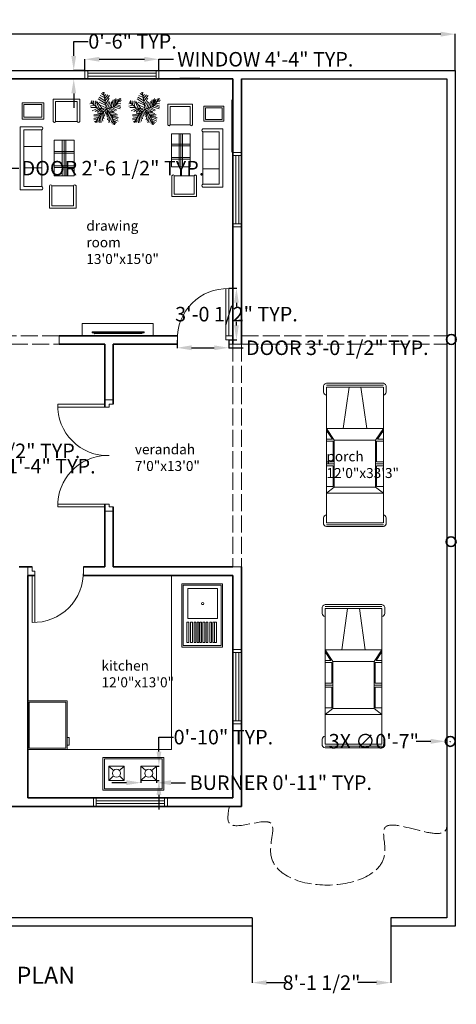
# Model space of a CAD drawing. Units: inches. Extents: x 29 to 4581, y 6 to 2196.
# Tile 3 of 3: x 4274 to 4581, y 1506 to 2196. Entities that reach past the tile are written whole.
import ezdxf

# ---------------------------------------------------------------- set-up
doc = ezdxf.new("R2010")
doc.units = ezdxf.units.IN
doc.header["$MEASUREMENT"] = 0
doc.linetypes.add('ACAD_ISO02W100', pattern=[15, 12, -3])
for name, color, linetype, lineweight in [('A-ANNO-DIMS', 2, 'Continuous', 18), ('A-ANNO-TEXT', 7, 'Continuous', 25), ('A-DOOR', 3, 'Continuous', 18), ('A-EQPM', 9, 'Continuous', 18), ('A-FLOR-CASE', 8, 'Continuous', 18), ('A-FLOR-FIXT', 9, 'Continuous', 18), ('A-GLAZ', 4, 'Continuous', 18), ('A-ROOF-OVHD', 8, 'ACAD_ISO02W100', 18), ('A-WALL', 7, 'Continuous', 35), ('A-WALL-OVHD', 8, 'ACAD_ISO02W100', 18), ('C-PKNG-VEHI', 8, 'Continuous', 13), ('C-PROP', 8, 'Continuous', 25), ('L-PLNT', 3, 'Continuous', 13)]:
    doc.layers.add(name, color=color, linetype=linetype, lineweight=lineweight)
for name, color, linetype, lineweight, true_color in [('A-AREA-IDEN', 41, 'Continuous', 18, 0xf4ee51), ('A-COLS', 240, 'Continuous', 35, 0xed1f24), ('A-FURN', 31, 'Continuous', 18, 0xfecc66)]:
    doc.layers.add(name, color=color, linetype=linetype, lineweight=lineweight, true_color=true_color)
doc.styles.get("Standard").update_dxf_attribs({"font": 'arial.ttf'})
doc.dimstyles.get("Standard").update_dxf_attribs({"dimtxt": 10.18, "dimasz": 10.18, "dimexe": 0.18, "dimexo": 0.0625, "dimgap": 0.09, "dimtad": 0, "dimtih": 1, "dimtoh": 1, "dimdec": 0, "dimzin": 0, "dimdsep": 46, "dimlunit": 3, "dimtxsty": 'Standard', "dimcen": 0.09, "dimadec": 0, "dimazin": 0, "dimtfac": 1, "dimtdec": 0, "dimtofl": 0, "dimtmove": 0, "dimatfit": 3, "dimfxl": 1, "dimtolj": 1, "dimtzin": 0, "dimarcsym": 0})

# ---------------------------------------------------------------- blocks, each defined once
blk = doc.blocks.new('*U4')
for p, q in [((-3.665, 19.273), (-27.574, 35.527)), ((-5.114, 28.097), (-24.676, 40.636)), ((-7.288, 39.707), (-21.778, 46.673)), ((-8.737, 47.138), (-17.069, 52.711)), ((-10.186, 53.64), (-13.084, 55.962)), ((0, 0), (-10.5, 57)), ((-9.099, 51.782), (-6.563, 55.962)), ((-7.65, 43.423), (-2.578, 49.46)), ((-5.839, 35.992), (4.667, 48.067)), ((-5.114, 27.632), (10.463, 46.673)), ((-2.941, 16.486), (8.652, 37.85)), ((27, 9), (48, 36)), ((27.127, 9.056), (31.112, 35.992)), ((38.719, 34.134), (41.979, 28.561)), ((44.153, 36.456), (45.239, 32.741)), ((-47.498, 19.737), (-55.83, 18.344)), ((-40.615, 13.7), (-55.105, 10.913)), ((-31.5, 4.5), (-52.5, 25.5)), ((-33.37, 6.269), (-52.207, 5.34)), ((-48.585, 21.131), (-49.309, 29.026)), ((-28.299, 3.483), (-47.86, -5.805)), ((-43.513, 28.561), (-42.427, 15.558)), ((-38.442, 26.239), (-34.819, 7.663)), ((-21.416, 3.018), (-38.079, -8.128)), ((-35.544, 28.097), (-24.314, 3.947)), ((0, 0), (-31.5, 4.5)), ((-14.533, 2.09), (-30.834, 25.31)), ((-15.982, 2.09), (-30.11, -9.521)), ((-24.314, 23.917), (-2.941, 13.7)), ((0, 0), (-22.5, -19.5)), ((-6.563, 1.161), (-21.416, -8.128)), ((-20.691, 13.7), (-1.129, 4.876)), ((-1.129, 6.734), (9.014, 26.704)), ((0, 0), (27, 9)), ((0, 0), (18, -22.5)), ((3.942, 1.625), (11.187, 24.381)), ((6.478, 1.625), (26.04, -8.592)), ((10.101, 3.483), (17.708, 26.239)), ((11.187, 3.483), (30.749, -5.805)), ((16.259, 5.805), (23.142, 31.348)), ((18.07, 5.805), (35.096, -3.483)), ((22.055, 7.198), (27.489, 32.277)), ((24.229, 7.663), (46.688, 1.625)), ((29.662, 12.307), (48.137, 6.269)), ((31.836, 30.883), (32.561, 16.486)), ((33.285, 16.486), (48.862, 10.913)), ((35.096, 32.741), (37.27, 22.524)), ((36.183, 19.737), (48.137, 17.88)), ((40.53, 25.775), (48.862, 24.846)), ((43.791, 29.954), (51.036, 30.883)), ((-17.431, -15.094), (-42.789, -18.809)), ((-28.299, -29.026), (-42.789, -31.348)), ((-24.314, -21.596), (-42.427, -22.06)), ((-26.849, -26.24), (-40.253, -25.775)), ((-22.5, -19.5), (-37.5, -45)), ((-15.257, -12.772), (-30.11, -12.772)), ((-29.023, -30.884), (-27.936, -43.887)), ((-25.038, -23.918), (-22.865, -45.281)), ((-20.691, -18.345), (-17.793, -44.352)), ((-6.563, -5.805), (-19.967, -9.985)), ((-17.069, -15.094), (-12.721, -40.172)), ((-13.446, -11.378), (-8.737, -32.741)), ((-9.461, -8.592), (-6.201, -23.453)), ((-4.752, -3.483), (-3.665, -14.629)), ((2.493, -3.019), (-1.491, -20.202)), ((1.769, -2.555), (24.229, -9.521)), ((5.029, -6.27), (2.131, -25.775)), ((9.014, -11.378), (3.58, -35.992)), ((14.085, -16.951), (6.478, -40.172)), ((7.565, -9.056), (32.198, -14.629)), ((18.07, -22.524), (8.289, -45.745)), ((12.274, -15.094), (36.907, -18.809)), ((20.244, -30.419), (15.897, -44.816)), ((16.259, -19.738), (36.183, -22.989)), ((18, -22.5), (27, -52.5)), ((18.433, -22.524), (40.53, -29.026)), ((19.157, -25.311), (38.719, -33.206)), ((21.331, -32.741), (39.081, -40.636)), ((-30.834, -34.135), (-42.427, -35.528)), ((-34.457, -39.708), (-40.978, -42.494)), ((-32.646, -36.921), (-31.921, -44.352)), ((22.78, -37.85), (19.519, -48.532)), ((22.78, -38.314), (34.372, -44.816)), ((24.591, -45.745), (23.142, -50.854)), ((24.591, -43.423), (30.749, -47.603)), ((26.764, -49.925), (28.213, -50.854))]:
    blk.add_line(p, q)
blk = doc.blocks.new('*U6')
for p, q in [((5.4, 42.3), (12.1, 42.3)), ((189.7, 42.3), (183, 42.3)), ((0.1, -0.4), (0.1, 38.3)), ((2.8, -0.4), (2.8, 38.3)), ((5.4, 38.3), (16.1, 38.3)), ((5.4, -0.4), (5.4, 38.2)), ((16.1, 38.3), (180.3, 38.3)), ((61.5, -0.4), (61.5, 38.3)), ((61.5, 38.3), (77.5, 27.6)), ((64.2, 38.3), (76.2, 30.3)), ((76.2, 30.3), (76.2, 38.3)), ((77.5, 27.6), (141.6, 27.6)), ((77.5, -0.4), (77.5, 27.6)), ((78.9, 38.3), (78.9, 29)), ((78.9, 29), (106.9, 29)), ((106.9, 29), (106.9, 38.3)), ((109.6, 27.6), (109.6, 38.3)), ((112.3, 38.3), (112.3, 29)), ((112.3, 29), (140.3, 29)), ((140.3, 29), (140.3, 38.3)), ((141.6, 27.6), (149.6, 38.3)), ((141.6, -0.4), (141.6, 27.6)), ((149.6, -0.4), (149.6, 38.3)), ((189.7, 38.3), (179, 38.3)), ((189.7, -0.4), (189.7, 38.2)), ((192.4, -0.4), (192.4, 38.3)), ((195, -0.4), (195, 38.3)), ((5.4, 7.6), (61.5, 15.6)), ((0.1, -0.4), (0.1, -39.2)), ((2.8, -0.4), (2.8, -39.1)), ((5.4, -0.4), (5.4, -39.1)), ((5.4, -8.4), (61.5, -16.4)), ((61.5, -0.4), (61.5, -39.1)), ((77.5, -0.4), (77.5, -28.5)), ((141.6, -0.4), (141.6, -28.5)), ((149.6, -0.4), (149.6, -39.1)), ((189.7, -0.4), (189.7, -39.1)), ((192.4, -0.4), (192.4, -39.1)), ((195, -0.4), (195, -39.2)), ((5.4, -39.1), (16.1, -39.1)), ((16.1, -39.1), (180.3, -39.1)), ((61.5, -39.1), (77.5, -28.5)), ((64.2, -39.1), (76.2, -31.1)), ((76.2, -31.1), (76.2, -39.1)), ((77.5, -28.5), (141.6, -28.5)), ((78.9, -39.1), (78.9, -29.8)), ((78.9, -29.8), (106.9, -29.8)), ((106.9, -29.8), (106.9, -39.1)), ((109.6, -28.5), (109.6, -39.1)), ((112.3, -29.8), (140.3, -29.8)), ((112.3, -39.1), (112.3, -29.8)), ((140.3, -29.8), (140.3, -39.1)), ((141.6, -28.5), (149.6, -39.1)), ((189.7, -39.1), (179, -39.1)), ((5.4, -43.1), (12.1, -43.1)), ((189.7, -43.1), (183, -43.1))]:
    blk.add_line(p, q)
for centre, radius, start, end in [((5.1, 37.3), 5.06, 85.6455, 168.0943), ((11.5, 37.6), 4.72, 8.1301, 81.87), ((183.7, 37.6), 4.72, 98.13, 171.8699), ((190.1, 37.3), 5.06, 11.9057, 94.3545), ((5.1, -38.1), 5.06, 191.9057, 274.3545), ((11.5, -38.5), 4.72, 278.13, 351.8699), ((183.7, -38.5), 4.72, 188.1301, 261.87), ((190.1, -38.1), 5.06, 265.6455, 348.0943)]:
    blk.add_arc(centre, radius, start, end)
blk = doc.blocks.new('*D7')
at = {"layer": 'A-ANNO-DIMS', "color": 0, "lineweight": -2, "transparency": 16777216}
for p, q in [((3871.98, 2160.26), (3871.98, 2185.77)), ((3882.16, 2185.59), (4217.25, 2185.59)), ((4569.8, 2185.59), (4234.7, 2185.59)), ((4579.98, 2160.26), (4579.98, 2185.77))]:
    blk.add_line(p, q, dxfattribs=at)
at = {"layer": 'A-ANNO-DIMS', "color": 0, "transparency": 16777216}
for points in [[(3882.16, 2187.28), (3882.16, 2183.89), (3871.98, 2185.59)], [(4569.8, 2187.28), (4569.8, 2183.89), (4579.98, 2185.59)]]:
    blk.add_solid(points, dxfattribs=at)
at = {"layer": 'Defpoints', "color": 0, "transparency": 16777216}
for p in [(4579.98, 2185.59), (3871.98, 2160.2), (4579.98, 2160.2)]:
    blk.add_point(p, dxfattribs=at)
at = {"layer": 'A-ANNO-DIMS', "color": 0, "transparency": 16777216, "insert": (4225.98, 2185.59), "char_height": 10.18, "attachment_point": 5}
blk.add_mtext("\\A1;59'", dxfattribs=at)
blk = doc.blocks.new('DOOR-36IN')
for p, q in [((34.01, 0), (34.01, 36)), ((36.01, 3), (36.01, 36)), ((34.01, 0), (36.01, 0))]:
    blk.add_line(p, q)
blk.add_arc((35.01, 1), 35.01, 88.36342, 181.63658)
blk = doc.blocks.new('DOOR-36IN-PAIRED-LEAF')
for p, q in [((36.01, 2), (0.01, 2)), ((36.01, 2), (36.01, 0)), ((33.01, 0), (0.01, 0))]:
    blk.add_line(p, q)
blk.add_arc((35.01, 1), 35.01, 91.63658, 181.63658)
blk = doc.blocks.new('WIN-48')
for p, q in [((0, 6), (0, 0)), ((2, 6), (2, 0)), ((2, 4), (50, 4)), ((2, 2), (50, 2)), ((50, 6), (50, 0)), ((52, 6), (52, 0))]:
    blk.add_line(p, q)
blk = doc.blocks.new('HOB-BURNER')
for p, q in [((0, 9.96), (3.37, 6.89)), ((10.94, 9.96), (7.57, 6.89)), ((0, 0), (3.37, 3.07)), ((10.94, 0), (7.57, 3.07))]:
    blk.add_line(p, q)
blk.add_lwpolyline([(0, 9.96), (10.94, 9.96), (10.94, 0), (0, 0)], close=True)
blk.add_circle((5.47, 4.98), 2.84)
blk = doc.blocks.new('PORCH-POST-ROUND')
blk.add_circle((3.47, 3.47), 3.47)
blk = doc.blocks.new('*D22')
at = {"layer": 'A-ANNO-DIMS', "color": 0, "lineweight": -2, "transparency": 16777216}
for p, q in [((4226.82, 1911.89), (4226.82, 1922.07)), ((4229.23, 1901.71), (4226.64, 1901.71)), ((4229.23, 1885.22), (4226.64, 1885.22)), ((4226.82, 1875.04), (4226.82, 1864.86))]:
    blk.add_line(p, q, dxfattribs=at)
at = {"layer": 'A-ANNO-DIMS', "color": 0, "transparency": 16777216}
for points in [[(4225.13, 1911.89), (4228.52, 1911.89), (4226.82, 1901.71)], [(4225.13, 1875.04), (4228.52, 1875.04), (4226.82, 1885.22)]]:
    blk.add_solid(points, dxfattribs=at)
at = {"layer": 'Defpoints', "color": 0, "transparency": 16777216}
for p in [(4229.3, 1901.71), (4226.82, 1885.22), (4229.3, 1885.22)]:
    blk.add_point(p, dxfattribs=at)
at = {"layer": 'A-ANNO-DIMS', "color": 0, "transparency": 16777216, "insert": (4226.82, 1893.47), "char_height": 10.18, "attachment_point": 5}
blk.add_mtext('\\A1;DINING CHAIR 1\'-4 1/2" TYP.', dxfattribs=at)
blk = doc.blocks.new('*D23')
at = {"layer": 'A-ANNO-DIMS', "color": 0, "lineweight": -2, "transparency": 16777216}
for p, q in [((4229.3, 1885.16), (4229.3, 1882.56)), ((4245.51, 1885.16), (4245.51, 1882.56)), ((4219.12, 1882.74), (4208.94, 1882.74)), ((4255.69, 1882.74), (4265.87, 1882.74))]:
    blk.add_line(p, q, dxfattribs=at)
at = {"layer": 'A-ANNO-DIMS', "color": 0, "transparency": 16777216}
for points in [[(4219.12, 1884.44), (4219.12, 1881.05), (4229.3, 1882.74)], [(4255.69, 1884.44), (4255.69, 1881.05), (4245.51, 1882.74)]]:
    blk.add_solid(points, dxfattribs=at)
at = {"layer": 'Defpoints', "color": 0, "transparency": 16777216}
for p in [(4229.3, 1885.22), (4245.51, 1885.22), (4245.51, 1882.74)]:
    blk.add_point(p, dxfattribs=at)
at = {"layer": 'A-ANNO-DIMS', "color": 0, "transparency": 16777216, "insert": (4296.5, 1882.74), "char_height": 10.18, "attachment_point": 5}
blk.add_mtext('\\A1;1\'-4" TYP.', dxfattribs=at)
blk = doc.blocks.new('*D24')
at = {"layer": 'A-ANNO-DIMS', "color": 0, "lineweight": -2, "transparency": 16777216}
for p, q in [((4384.7, 1971.13), (4384.7, 1965.58)), ((4420.98, 1971.13), (4420.98, 1965.58)), ((4394.88, 1965.76), (4410.8, 1965.76)), ((4420.98, 1965.76), (4431.16, 1965.76))]:
    blk.add_line(p, q, dxfattribs=at)
at = {"layer": 'A-ANNO-DIMS', "color": 0, "transparency": 16777216}
for points in [[(4394.88, 1967.45), (4394.88, 1964.06), (4384.7, 1965.76)], [(4410.8, 1967.45), (4410.8, 1964.06), (4420.98, 1965.76)]]:
    blk.add_solid(points, dxfattribs=at)
at = {"layer": 'Defpoints', "color": 0, "transparency": 16777216}
for p in [(4384.7, 1971.2), (4420.98, 1971.2), (4420.98, 1965.76)]:
    blk.add_point(p, dxfattribs=at)
at = {"layer": 'A-ANNO-DIMS', "color": 0, "transparency": 16777216, "insert": (4497.19, 1965.76), "char_height": 10.18, "attachment_point": 5}
blk.add_mtext('\\A1;DOOR 3\'-0 1/2" TYP.', dxfattribs=at)
blk = doc.blocks.new('*D25')
at = {"layer": 'A-ANNO-DIMS', "color": 0, "lineweight": -2, "transparency": 16777216}
for p, q in [((4421.04, 2007.47), (4426.6, 2007.47)), ((4426.42, 1997.29), (4426.42, 1994.69)), ((4426.42, 1981.38), (4426.42, 1983.98)), ((4421.04, 1971.2), (4426.6, 1971.2))]:
    blk.add_line(p, q, dxfattribs=at)
at = {"layer": 'A-ANNO-DIMS', "color": 0, "transparency": 16777216}
for points in [[(4424.72, 1997.29), (4428.11, 1997.29), (4426.42, 2007.47)], [(4424.72, 1981.38), (4428.11, 1981.38), (4426.42, 1971.2)]]:
    blk.add_solid(points, dxfattribs=at)
at = {"layer": 'Defpoints', "color": 0, "transparency": 16777216}
for p in [(4420.98, 2007.47), (4426.42, 2007.47), (4420.98, 1971.2)]:
    blk.add_point(p, dxfattribs=at)
at = {"layer": 'A-ANNO-DIMS', "color": 0, "transparency": 16777216, "insert": (4426.42, 1989.33), "char_height": 10.18, "attachment_point": 5}
blk.add_mtext('\\A1;3\'-0 1/2" TYP.', dxfattribs=at)
blk = doc.blocks.new('*D26')
at = {"layer": 'A-ANNO-DIMS', "color": 0, "lineweight": -2, "transparency": 16777216}
for p, q in [((4319.98, 2160.26), (4319.98, 2168.18)), ((4330.16, 2168), (4361.8, 2168)), ((4371.98, 2160.26), (4371.98, 2168.18)), ((4371.98, 2168), (4382.16, 2168))]:
    blk.add_line(p, q, dxfattribs=at)
at = {"layer": 'A-ANNO-DIMS', "color": 0, "transparency": 16777216}
for points in [[(4330.16, 2169.69), (4330.16, 2166.3), (4319.98, 2168)], [(4361.8, 2169.69), (4361.8, 2166.3), (4371.98, 2168)]]:
    blk.add_solid(points, dxfattribs=at)
at = {"layer": 'Defpoints', "color": 0, "transparency": 16777216}
for p in [(4371.98, 2168), (4319.98, 2160.2), (4371.98, 2160.2)]:
    blk.add_point(p, dxfattribs=at)
at = {"layer": 'A-ANNO-DIMS', "color": 0, "transparency": 16777216, "insert": (4446.66, 2168), "char_height": 10.18, "attachment_point": 5}
blk.add_mtext('\\A1;WINDOW 4\'-4" TYP.', dxfattribs=at)
blk = doc.blocks.new('*D27')
at = {"layer": 'A-ANNO-DIMS', "color": 0, "lineweight": -2, "transparency": 16777216}
for p, q in [((4312.18, 2170.38), (4312.18, 2180.56)), ((4312.18, 2180.56), (4322.36, 2180.56)), ((4319.91, 2160.2), (4312, 2160.2)), ((4319.91, 2154.2), (4312, 2154.2)), ((4312.18, 2144.02), (4312.18, 2133.84))]:
    blk.add_line(p, q, dxfattribs=at)
at = {"layer": 'A-ANNO-DIMS', "color": 0, "transparency": 16777216}
for points in [[(4310.48, 2170.38), (4313.87, 2170.38), (4312.18, 2160.2)], [(4310.48, 2144.02), (4313.87, 2144.02), (4312.18, 2154.2)]]:
    blk.add_solid(points, dxfattribs=at)
at = {"layer": 'Defpoints', "color": 0, "transparency": 16777216}
for p in [(4312.18, 2160.2), (4319.98, 2160.2), (4319.98, 2154.2)]:
    blk.add_point(p, dxfattribs=at)
at = {"layer": 'A-ANNO-DIMS', "color": 0, "transparency": 16777216, "insert": (4353.47, 2180.56), "char_height": 10.18, "attachment_point": 5}
blk.add_mtext('\\A1;0\'-6" TYP.', dxfattribs=at)
blk = doc.blocks.new('*D28')
at = {"layer": 'A-ANNO-DIMS', "color": 0, "lineweight": -2, "transparency": 16777216}
for p, q in [((4263.52, 2081.47), (4263.52, 2091.65)), ((4263.52, 2091.65), (4273.7, 2091.65)), ((4259.04, 2081.47), (4263.7, 2081.47)), ((4263.52, 2061.38), (4263.52, 2071.29)), ((4259.04, 2051.2), (4263.7, 2051.2))]:
    blk.add_line(p, q, dxfattribs=at)
at = {"layer": 'A-ANNO-DIMS', "color": 0, "transparency": 16777216}
for points in [[(4261.82, 2071.29), (4265.21, 2071.29), (4263.52, 2081.47)], [(4261.82, 2061.38), (4265.21, 2061.38), (4263.52, 2051.2)]]:
    blk.add_solid(points, dxfattribs=at)
at = {"layer": 'Defpoints', "color": 0, "transparency": 16777216}
for p in [(4258.98, 2081.47), (4263.52, 2081.47), (4258.98, 2051.2)]:
    blk.add_point(p, dxfattribs=at)
at = {"layer": 'A-ANNO-DIMS', "color": 0, "transparency": 16777216, "insert": (4339.73, 2091.65), "char_height": 10.18, "attachment_point": 5}
blk.add_mtext('\\A1;DOOR 2\'-6 1/2" TYP.', dxfattribs=at)
blk = doc.blocks.new('*D44')
at = {"layer": 'A-ANNO-DIMS', "color": 0, "lineweight": -2, "transparency": 16777216}
for p, q in [((4349.23, 1660.87), (4339.05, 1660.87)), ((4359.41, 1662.45), (4359.41, 1660.69)), ((4370.35, 1662.45), (4370.35, 1660.69)), ((4380.53, 1660.87), (4390.71, 1660.87))]:
    blk.add_line(p, q, dxfattribs=at)
at = {"layer": 'A-ANNO-DIMS', "color": 0, "transparency": 16777216}
for points in [[(4349.23, 1662.57), (4349.23, 1659.18), (4359.41, 1660.87)], [(4380.53, 1662.57), (4380.53, 1659.18), (4370.35, 1660.87)]]:
    blk.add_solid(points, dxfattribs=at)
at = {"layer": 'Defpoints', "color": 0, "transparency": 16777216}
for p in [(4359.41, 1662.51), (4370.35, 1662.51), (4370.35, 1660.87)]:
    blk.add_point(p, dxfattribs=at)
at = {"layer": 'A-ANNO-DIMS', "color": 0, "transparency": 16777216, "insert": (4457.56, 1660.87), "char_height": 10.18, "attachment_point": 5}
blk.add_mtext('\\A1;BURNER 0\'-11" TYP.', dxfattribs=at)
blk = doc.blocks.new('*D45')
at = {"layer": 'A-ANNO-DIMS', "color": 0, "lineweight": -2, "transparency": 16777216}
for p, q in [((4371.99, 1682.65), (4371.99, 1692.83)), ((4371.99, 1692.83), (4382.17, 1692.83)), ((4370.41, 1672.47), (4372.17, 1672.47)), ((4370.41, 1662.51), (4372.17, 1662.51)), ((4371.99, 1652.33), (4371.99, 1642.15))]:
    blk.add_line(p, q, dxfattribs=at)
at = {"layer": 'A-ANNO-DIMS', "color": 0, "transparency": 16777216}
for points in [[(4370.29, 1682.65), (4373.69, 1682.65), (4371.99, 1672.47)], [(4370.29, 1652.33), (4373.69, 1652.33), (4371.99, 1662.51)]]:
    blk.add_solid(points, dxfattribs=at)
at = {"layer": 'Defpoints', "color": 0, "transparency": 16777216}
for p in [(4370.35, 1672.47), (4371.99, 1672.47), (4370.35, 1662.51)]:
    blk.add_point(p, dxfattribs=at)
at = {"layer": 'A-ANNO-DIMS', "color": 0, "transparency": 16777216, "insert": (4417.24, 1692.83), "char_height": 10.18, "attachment_point": 5}
blk.add_mtext('\\A1;0\'-10" TYP.', dxfattribs=at)
blk = doc.blocks.new('*D46')
at = {"layer": 'A-ANNO-DIMS', "color": 0, "lineweight": -2, "transparency": 16777216}
for p, q in [((4437.42, 1560.13), (4437.42, 1520.52)), ((4534.84, 1560.13), (4534.84, 1520.52)), ((4447.6, 1520.7), (4460.64, 1520.7)), ((4524.66, 1520.7), (4511.62, 1520.7))]:
    blk.add_line(p, q, dxfattribs=at)
at = {"layer": 'A-ANNO-DIMS', "color": 0, "transparency": 16777216}
for points in [[(4447.6, 1522.39), (4447.6, 1519), (4437.42, 1520.7)], [(4524.66, 1522.39), (4524.66, 1519), (4534.84, 1520.7)]]:
    blk.add_solid(points, dxfattribs=at)
at = {"layer": 'Defpoints', "color": 0, "transparency": 16777216}
for p in [(4437.42, 1560.2), (4534.84, 1560.2), (4534.84, 1520.7)]:
    blk.add_point(p, dxfattribs=at)
at = {"layer": 'A-ANNO-DIMS', "color": 0, "transparency": 16777216, "insert": (4486.13, 1520.7), "char_height": 10.18, "attachment_point": 5}
blk.add_mtext('\\A1;8\'-1 1/2"', dxfattribs=at)
blk = doc.blocks.new('*D50')
at = {"layer": 'A-ANNO-DIMS', "color": 0, "lineweight": -2, "transparency": 16777216}
for p, q in [((4552.67, 1689.94), (4562.85, 1689.89)), ((4576.41, 1689.82), (4576.59, 1689.82)), ((4576.5, 1689.73), (4576.5, 1689.91))]:
    blk.add_line(p, q, dxfattribs=at)
at = {"layer": 'A-ANNO-DIMS', "color": 0, "transparency": 16777216}
blk.add_solid([(4562.86, 1691.59), (4562.85, 1688.19), (4573.03, 1689.84)], dxfattribs=at)
at = {"layer": 'Defpoints', "color": 0, "transparency": 16777216}
for p in [(4573.03, 1689.84), (4579.97, 1689.81)]:
    blk.add_point(p, dxfattribs=at)
at = {"layer": 'A-ANNO-DIMS', "color": 0, "transparency": 16777216, "insert": (4522.85, 1689.94), "char_height": 10.18, "attachment_point": 5}
blk.add_mtext('\\A1;3X ∅0\'-7"', dxfattribs=at)

msp = doc.modelspace()

# ---------------------------------------------------------------- linework, layer by layer
at = {"layer": 'A-DOOR'}
for p, q in [((4384.98, 1974.2), (4384.98, 1968.2)), ((4418.98, 1974.2), (4423.98, 1974.2)), ((4420.98, 1971.2), (4420.98, 1968.2)), ((4420.98, 1968.2), (4423.98, 1968.2)), ((4339.98, 1929.2), (4333.98, 1929.2)), ((4339.98, 1926.2), (4336.98, 1926.2)), ((4333.98, 1890.24), (4333.98, 1890.15)), ((4336.98, 1890.2), (4333.98, 1890.2)), ((4339.98, 1851.2), (4333.98, 1851.2)), ((4339.98, 1854.2), (4336.98, 1854.2)), ((4279.98, 1806.2), (4279.98, 1812.2)), ((4282.98, 1809.2), (4282.98, 1812.2)), ((4318.98, 1806.2), (4318.98, 1812.2))]:
    msp.add_line(p, q, dxfattribs=at)
at = {"layer": 'A-EQPM'}
for p, q in [((4327.52, 1976.14), (4326.64, 1975.61)), ((4326.64, 1975.61), (4360.24, 1975.67)), ((4360.24, 1975.67), (4359.23, 1976.14))]:
    msp.add_line(p, q, dxfattribs=at)
for points in [[(4318.17, 1974.2), (4368.06, 1974.2), (4368.06, 1982.86), (4318.17, 1982.86)], [(4325.24, 1976.99), (4361.61, 1976.99), (4361.61, 1976.14), (4325.24, 1976.14)], [(4279.98, 1718.34), (4307.57, 1718.34), (4307.57, 1684.14), (4279.98, 1684.14)], [(4280.98, 1717.34), (4306.57, 1717.34), (4306.57, 1685.14), (4280.98, 1685.14)], [(4307.57, 1687.9), (4307.57, 1687.9), (4307.57, 1694.82), (4307.57, 1694.82)], [(4307.57, 1687.15), (4309.1, 1687.15), (4309.1, 1692.45), (4307.57, 1692.45)], [(4332.73, 1678.63), (4375.37, 1678.63), (4375.37, 1655.6), (4332.73, 1655.6)], [(4333.73, 1677.63), (4374.37, 1677.63), (4374.37, 1656.6), (4333.73, 1656.6)]]:
    msp.add_lwpolyline(points, close=True, dxfattribs=at)
at = {"layer": 'A-FLOR-CASE'}
for p, q in [((4380.83, 1806.2), (4380.83, 1684.14)), ((4380.83, 1684.14), (4279.98, 1684.14))]:
    msp.add_line(p, q, dxfattribs=at)
at = {"layer": 'A-FLOR-FIXT'}
for points in [[(4416.67, 1800.35), (4388.04, 1800.35), (4388.04, 1755.97), (4416.67, 1755.97)], [(4415.67, 1799.35), (4389.04, 1799.35), (4389.04, 1756.97), (4415.67, 1756.97)], [(4392.31, 1796.95), (4413, 1796.95), (4413, 1775.95), (4392.31, 1775.95)], [(4392.9, 1773.39), (4391.67, 1773.39), (4391.67, 1759.08), (4392.9, 1759.08)], [(4395.46, 1773.39), (4394.23, 1773.39), (4394.23, 1759.08), (4395.46, 1759.08)], [(4397.88, 1773.39), (4396.65, 1773.39), (4396.65, 1759.08), (4397.88, 1759.08)], [(4400, 1773.39), (4398.76, 1773.39), (4398.76, 1759.08), (4400, 1759.08)], [(4401.93, 1773.39), (4400.7, 1773.39), (4400.7, 1759.08), (4401.93, 1759.08)], [(4404.13, 1773.39), (4402.9, 1773.39), (4402.9, 1759.08), (4404.13, 1759.08)], [(4406.38, 1773.39), (4405.15, 1773.39), (4405.15, 1759.08), (4406.38, 1759.08)], [(4408.97, 1773.39), (4407.74, 1773.39), (4407.74, 1759.08), (4408.97, 1759.08)], [(4411.09, 1773.39), (4409.85, 1773.39), (4409.85, 1759.08), (4411.09, 1759.08)], [(4412.32, 1773.39), (4411.09, 1773.39), (4411.09, 1759.08), (4412.32, 1759.08)]]:
    msp.add_lwpolyline(points, close=True, dxfattribs=at)
msp.add_circle((4402.65, 1786.45), 0.779, dxfattribs=at)
at = {"layer": 'A-FURN'}
for p, q in [((4386.19, 2115.79), (4386.19, 2092.65)), ((4387.37, 2115.79), (4387.37, 2092.65)), ((4388.55, 2115.79), (4388.55, 2092.65)), ((4277.28, 2106.91), (4289.76, 2106.91)), ((4304.14, 2111.39), (4304.14, 2086.31)), ((4305.42, 2111.39), (4305.42, 2086.31)), ((4306.69, 2111.39), (4306.69, 2086.31)), ((4380.91, 2108.42), (4393.84, 2108.42)), ((4380.91, 2107.24), (4393.84, 2107.24)), ((4298.4, 2103.4), (4312.43, 2103.4)), ((4298.4, 2102.12), (4312.43, 2102.12)), ((4380.91, 2099.19), (4393.84, 2099.19)), ((4414.38, 2105.01), (4402.87, 2105.01)), ((4277.28, 2091.85), (4289.76, 2091.85)), ((4298.4, 2093.39), (4312.43, 2093.39)), ((4298.4, 2092.11), (4312.43, 2092.11)), ((4380.91, 2098.01), (4393.84, 2098.01)), ((4414.38, 2091.11), (4402.87, 2091.11))]:
    msp.add_line(p, q, dxfattribs=at)
for points in [[(4386.64, 2154.72), (4400.72, 2154.72)], [(4297.76, 2124.44), (4297.76, 2140.05), (4299.44, 2140.05)], [(4314.7, 2140.05), (4299.44, 2140.05)], [(4314.7, 2140.05), (4316.37, 2140.05), (4316.37, 2124.44)], [(4299.44, 2138.42), (4299.44, 2124.44), (4299.43, 2124.44)], [(4314.7, 2124.44), (4314.7, 2138.42)], [(4378.31, 2122.06), (4378.31, 2136.46), (4379.85, 2136.46)], [(4379.85, 2134.95), (4379.85, 2122.06), (4379.84, 2122.06)], [(4393.93, 2136.46), (4379.85, 2136.46)], [(4393.93, 2136.46), (4395.47, 2136.46), (4395.47, 2122.06)], [(4393.93, 2122.06), (4393.93, 2134.95)], [(4423.22, 2139.62), (4423.22, 2102.98)], [(4289.7, 2120.73), (4274.51, 2120.73), (4274.51, 2118.5)], [(4416.94, 2117.11), (4416.94, 2119.16), (4402.93, 2119.16)], [(4274.51, 2118.5), (4274.51, 2078.78)], [(4277.28, 2118.5), (4289.7, 2118.5)], [(4416.94, 2080.42), (4416.94, 2117.07)], [(4382.7, 2071.85), (4381.16, 2071.85), (4381.16, 2086.25)], [(4382.7, 2086.25), (4382.7, 2073.36)], [(4398.33, 2086.25), (4398.33, 2071.85), (4396.79, 2071.85)], [(4396.79, 2073.36), (4396.79, 2086.25), (4396.79, 2086.25)], [(4274.51, 2078.73), (4274.51, 2076.5), (4289.7, 2076.5)], [(4296.87, 2063.71), (4295.2, 2063.71), (4295.2, 2079.32)], [(4296.87, 2079.32), (4296.87, 2065.34)], [(4313.81, 2079.32), (4313.81, 2063.71), (4312.14, 2063.71)], [(4312.14, 2065.34), (4312.14, 2079.32), (4312.14, 2079.32)], [(4402.93, 2078.37), (4416.94, 2078.37), (4416.94, 2080.42)], [(4414.38, 2080.42), (4402.93, 2080.42)], [(4396.79, 2073.36), (4382.7, 2073.36)], [(4382.7, 2071.85), (4396.79, 2071.85)], [(4312.14, 2065.34), (4296.87, 2065.34)], [(4296.87, 2063.71), (4312.14, 2063.71)]]:
    msp.add_lwpolyline(points, dxfattribs=at)
for points in [[(4275.91, 2137.57), (4291.15, 2137.57), (4291.15, 2126.06), (4275.91, 2126.06)], [(4277.19, 2136.29), (4289.88, 2136.29), (4289.88, 2127.34), (4277.19, 2127.34)], [(4299.44, 2138.42), (4314.67, 2138.42), (4314.67, 2124.48), (4299.44, 2124.48)], [(4379.85, 2134.95), (4393.9, 2134.95), (4393.9, 2122.1), (4379.85, 2122.1)], [(4403.55, 2135.19), (4417.61, 2135.19), (4417.61, 2124.57), (4403.55, 2124.57)], [(4404.73, 2134.01), (4416.43, 2134.01), (4416.43, 2125.75), (4404.73, 2125.75)], [(4289.76, 2118.5), (4277.28, 2118.5), (4277.28, 2078.76), (4289.76, 2078.76)], [(4380.91, 2115.79), (4393.84, 2115.79), (4393.84, 2092.65), (4380.91, 2092.65)], [(4402.87, 2080.42), (4414.38, 2080.42), (4414.38, 2117.08), (4402.87, 2117.08)], [(4298.4, 2111.39), (4312.43, 2111.39), (4312.43, 2086.31), (4298.4, 2086.31)], [(4396.79, 2073.36), (4382.73, 2073.36), (4382.73, 2086.22), (4396.79, 2086.22)], [(4312.14, 2065.34), (4296.9, 2065.34), (4296.9, 2079.28), (4312.14, 2079.28)]]:
    msp.add_lwpolyline(points, close=True, dxfattribs=at)
for centre, radius, start, end in [((4289.45, 2119.6), 1.15, 285.56703, 77.60297), ((4298.6, 2124.6), 0.847, 190.55771, 7.81417), ((4315.54, 2124.61), 0.853, 191.62497, 348.37503), ((4379.07, 2122.21), 0.781, 190.55771, 7.81417), ((4394.7, 2122.22), 0.787, 191.62497, 348.37503), ((4403.34, 2118.14), 1.11, 112.09506, 247.90494), ((4381.93, 2086.09), 0.787, 11.62497, 168.37503), ((4397.56, 2086.11), 0.781, 10.55771, 187.81417), ((4289.25, 2077.62), 1.2, 292.09506, 67.90494), ((4296.04, 2079.15), 0.853, 11.62497, 168.37503), ((4312.98, 2079.16), 0.847, 10.55771, 187.81417), ((4403.15, 2079.4), 1.06, 105.56703, 257.60297)]:
    msp.add_arc(centre, radius, start, end, dxfattribs=at)
at = {"layer": 'A-ROOF-OVHD'}
for p, q in [((4429.98, 1974.2), (4573.98, 1974.2)), ((4423.98, 1968.2), (4429.98, 1968.2)), ((4423.98, 1968.2), (4423.98, 1812.2)), ((4429.98, 1968.2), (4429.98, 1812.2)), ((4429.98, 1968.2), (4573.98, 1968.2)), ((4423.98, 1812.2), (4429.98, 1812.2))]:
    msp.add_line(p, q, dxfattribs=at)
msp.add_open_spline([(4421.39, 1644.2), (4420.54, 1639.48), (4417.59, 1623.01), (4459.92, 1643.55), (4433.58, 1580.96), (4544.01, 1582.23), (4521.43, 1645.35), (4575.58, 1614.88), (4574.13, 1632.47), (4573.98, 1634.34)], degree=3, knots=[0, 0, 0, 0, 11.69459, 40.776133, 61.753444, 141.826335, 159.498194, 202.927614, 208.068359, 208.068359, 208.068359, 208.068359], dxfattribs=at)
at = {"layer": 'A-WALL'}
for p, q in [((4267.98, 2154.2), (4423.98, 2154.2)), ((4423.98, 2154.2), (4423.98, 1968.2)), ((4429.98, 2154.2), (4429.98, 1968.2)), ((4302.01, 1974.2), (4385.02, 1974.2)), ((4302.01, 1968.2), (4333.98, 1968.2)), ((4333.98, 1968.2), (4333.98, 1924.2)), ((4339.98, 1968.2), (4339.98, 1926.2)), ((4339.98, 1968.2), (4384.98, 1968.2)), ((4333.98, 1856.2), (4333.98, 1812.2)), ((4339.98, 1854.2), (4339.98, 1812.2)), ((4273.98, 1812.2), (4282.98, 1812.2)), ((4318.98, 1812.2), (4333.98, 1812.2)), ((4339.98, 1812.2), (4423.98, 1812.2)), ((4429.98, 1812.2), (4429.98, 1644.2)), ((4279.98, 1806.2), (4279.98, 1650.2)), ((4279.98, 1806.2), (4284.98, 1806.2)), ((4318.93, 1806.2), (4423.98, 1806.2)), ((4423.98, 1806.2), (4423.98, 1650.2)), ((4279.98, 1650.2), (4423.98, 1650.2)), ((4198.98, 1644.2), (4429.98, 1644.2))]:
    msp.add_line(p, q, dxfattribs=at)
at = {"layer": 'A-WALL-OVHD'}
for p, q in [((4302.01, 1974.2), (4267.98, 1974.2)), ((4302.01, 1974.2), (4302.01, 1968.2)), ((4267.98, 1968.2), (4302.01, 1968.2))]:
    msp.add_line(p, q, dxfattribs=at)
at = {"layer": 'C-PROP'}
for p, q in [((3871.98, 2160.2), (4579.98, 2160.2)), ((4429.98, 2154.2), (4573.98, 2154.2)), ((4573.98, 2154.2), (4573.98, 1566.2)), ((4579.98, 2160.2), (4579.98, 1560.2)), ((4573.98, 1968.2), (4573.98, 1812.2)), ((4573.98, 1806.2), (4573.98, 1566.2)), ((4437.42, 1560.2), (3871.98, 1560.2)), ((4437.42, 1566.2), (3877.98, 1566.2)), ((4437.42, 1566.2), (4437.42, 1560.2)), ((4573.98, 1566.2), (4534.84, 1566.2)), ((4534.84, 1566.2), (4534.84, 1560.2)), ((4579.98, 1560.2), (4534.84, 1560.2))]:
    msp.add_line(p, q, dxfattribs=at)

# ---------------------------------------------------------------- block references
at = {"layer": 'A-COLS'}
for p in [(4573.82, 1968.12), (4573.6, 1826.34), (4573.03, 1686.35)]:
    msp.add_blockref('PORCH-POST-ROUND', p, dxfattribs=at)
at = {"layer": 'A-DOOR'}
for name, p in [('DOOR-36IN', (4384.96, 1971.2)), ('DOOR-36IN-PAIRED-LEAF', (4300.96, 1854.2))]:
    msp.add_blockref(name, p, dxfattribs=at)
for p, rotation in [((4336.98, 1890.18), 90.00000000000207), ((4318.99, 1809.2), 180)]:
    msp.add_blockref('DOOR-36IN', p, dxfattribs=dict(at, rotation=rotation))
at = {"layer": 'A-EQPM'}
for p in [(4336.76, 1662.51), (4359.41, 1662.51)]:
    msp.add_blockref('HOB-BURNER', p, dxfattribs=at)
at = {"layer": 'A-GLAZ'}
for p in [(4319.98, 2154.2), (4325.98, 1644.2)]:
    msp.add_blockref('WIN-48', p, dxfattribs=at)
for p, rotation in [((4429.98, 2050.54), 89.99999999999837), ((4429.98, 1702.2), 89.99999999999628)]:
    msp.add_blockref('WIN-48', p, dxfattribs=dict(at, rotation=rotation))
at = {"layer": 'C-PKNG-VEHI', "xscale": 0.5158566261171222, "yscale": 0.5158566261171222, "zscale": 0.5158566261171222, "rotation": 270}
for p in [(4509.78, 1940.98), (4508.8, 1785.81)]:
    msp.add_blockref('*U6', p, dxfattribs=at)
at = {"layer": 'L-PLNT', "xscale": 0.2082080613586284, "yscale": 0.2082080613586284, "zscale": 0.2082080613586284}
for p in [(4335.17, 2132.96), (4362.38, 2132.96)]:
    msp.add_blockref('*U4', p, dxfattribs=at)

# ---------------------------------------------------------------- texts
at = {"layer": 'A-ANNO-TEXT', "insert": (4143.39, 1531.88), "char_height": 12, "attachment_point": 1}
msp.add_mtext_dynamic_manual_height_columns('GROUND FLOOR PLAN', width=542.8499, gutter_width=1, heights=[0], dxfattribs=at)
at = {"layer": 'A-AREA-IDEN', "char_height": 7, "attachment_point": 1}
for s, insert in [('drawing room\\P13\'0"x15\'0"', (4321.04, 2054.82)), ('verandah\\P7\'0"x13\'0"', (4355.13, 1898.06)), ('porch\\P12\'0"x33\'3"', (4489.59, 1893.12)), ('kitchen\\P12\'0"x13\'0"', (4331.69, 1746.42))]:
    msp.add_mtext_dynamic_manual_height_columns(s, width=59.5635, gutter_width=1, heights=[0], dxfattribs=dict(at, insert=insert))

# ---------------------------------------------------------------- dimensions: what is measured, and where the dimension line sits
at = {"layer": 'A-ANNO-DIMS'}
for base, p1, p2, angle, text, picture, middle in [((4312.18, 2160.2), (4319.98, 2154.2), (4319.98, 2160.2), 90, '<> TYP.', '*D27', (4353.47, 2180.56)), ((4263.52, 2081.47), (4258.98, 2051.2), (4258.98, 2081.47), 90, 'DOOR <> TYP.', '*D28', (4339.73, 2091.65)), ((4426.42, 2007.47), (4420.98, 1971.2), (4420.98, 2007.47), 90, '<> TYP.', '*D25', (4426.42, 1989.33)), ((4226.82, 1885.22), (4229.3, 1901.71), (4229.3, 1885.22), 270, 'DINING CHAIR <> TYP.', '*D22', (4226.82, 1893.47)), ((4245.51, 1882.74), (4229.3, 1885.22), (4245.51, 1885.22), 0, '<> TYP.', '*D23', (4296.5, 1882.74)), ((4371.99, 1672.47), (4370.35, 1662.51), (4370.35, 1672.47), 90, '<> TYP.', '*D45', (4417.24, 1692.83))]:
    dim = msp.add_linear_dim(base=base, p1=p1, p2=p2, angle=angle, text=text, dimstyle='Standard', override={"dimdec": 1, "dimlfac": 1, "dimrnd": 0, "dimzin": 1, "dimdsep": 46, "dimlunit": 4, "dimfrac": 2}, dxfattribs=at)
    dim.commit()
    dim.dimension.update_dxf_attribs({"geometry": picture, "text_midpoint": middle})
for base, p1, p2, override, picture, middle in [((4579.98, 2185.59), (3871.98, 2160.2), (4579.98, 2160.2), {"dimclrd": 0, "dimclre": 0, "dimclrt": 0}, '*D7', (4225.98, 2185.59)), ((4534.84, 1520.7), (4437.42, 1560.2), (4534.84, 1560.2), {"dimdec": 1, "dimlfac": 1, "dimrnd": 0, "dimzin": 1, "dimdsep": 46, "dimlunit": 4, "dimfrac": 2}, '*D46', (4486.13, 1520.7))]:
    dim = msp.add_linear_dim(base=base, p1=p1, p2=p2, dimstyle='Standard', override=override, dxfattribs=at)
    dim.commit()
    dim.dimension.update_dxf_attribs({"geometry": picture, "text_midpoint": middle})
for base, p1, p2, text, picture, middle in [((4371.98, 2168), (4319.98, 2160.2), (4371.98, 2160.2), 'WINDOW <> TYP.', '*D26', (4446.66, 2168)), ((4420.98, 1965.76), (4384.7, 1971.2), (4420.98, 1971.2), 'DOOR <> TYP.', '*D24', (4497.19, 1965.76)), ((4370.35, 1660.87), (4359.41, 1662.51), (4370.35, 1662.51), 'BURNER <> TYP.', '*D44', (4457.56, 1660.87))]:
    dim = msp.add_linear_dim(base=base, p1=p1, p2=p2, text=text, dimstyle='Standard', override={"dimdec": 1, "dimlfac": 1, "dimrnd": 0, "dimzin": 1, "dimdsep": 46, "dimlunit": 4, "dimfrac": 2}, dxfattribs=at)
    dim.commit()
    dim.dimension.update_dxf_attribs({"geometry": picture, "text_midpoint": middle})
dim = msp.add_diameter_dim_2p(p1=(4579.97, 1689.81), p2=(4573.03, 1689.84), text='3X <>', dimstyle='Standard', override={"dimdec": 1, "dimlfac": 1, "dimrnd": 0, "dimzin": 1, "dimdsep": 46, "dimlunit": 4, "dimfrac": 2}, dxfattribs=at)
dim.commit()
dim.dimension.update_dxf_attribs({"geometry": '*D50', "text_midpoint": (4552.67, 1689.94)})

doc.saveas('drawing.dxf')
